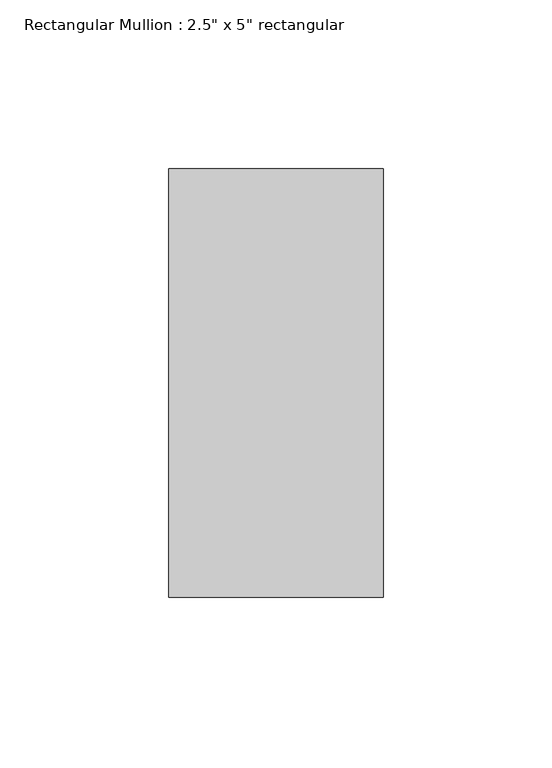
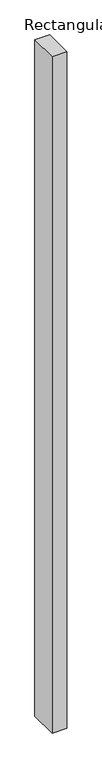
"""IFC4 building model written with IfcOpenShell, lengths in millimetres: member geometry."""

from ifc_helpers import new_model, si_unit, frame, origin, place, context, project, spatial, polyline, outline, extrude, source, transform, mapped, element, save


def member_eaba9652(model_context):
    return source(origin(), model_context, "Body", "SweptSolid", [
        extrude(outline(polyline([(31.75, 63.5), (31.75, -63.5), (-31.75, -63.5), (-31.75, 63.5), (31.75, 63.5)])), frame((0.0, 0.0, -3048.0), z_axis=(0.0, 0.0, 1.0), x_axis=(1.0, 0.0, 0.0)), (0.0, 0.0, 1.0), 3048.0),
    ])


if __name__ == "__main__":
    model = new_model("IFC4")
    model_context = context("Model", 3, world=origin())
    ifc_project = project(units=[si_unit("LENGTHUNIT", "METRE", prefix="MILLI")], contexts=[model_context])
    site = spatial("IfcSite", under=ifc_project)
    building = spatial("IfcBuilding", under=site)
    placement = place(None, origin())
    member_shape = member_eaba9652(model_context)
    element("IfcMember", 1, ObjectType="Rectangular Mullion : 2.5\" x 5\" rectangular", at=placement, inside=building, context=model_context, shape_type="MappedRepresentation", body=[
        mapped(member_shape, transform((0.0, 0.0, 0.0), x_axis=(1.0, 0.0, 0.0), y_axis=(0.0, 1.0, 0.0), z_axis=(0.0, 0.0, 1.0))),
    ])
    save(model, "model.ifc")

# Revit data of these elements
# Type "Rectangular Mullion : 2.5\" x 5\" rectangular"
#   built-in parameter 1007304 = 0.416667 (stored number, unit not read)
#   built-in parameter 1007301 = 0.104167 (stored number, unit not read)
#   built-in parameter 1007300 = 0.104167 (stored number, unit not read)
# Element 1 (IfcMember, "Rectangular Mullion : 2.5\" x 5\" rectangular")
#   Materials on its faces: "Aluminum"
# Materials
#   "Aluminum": class "Metal", colour RGB 247 247 247, transparency 0, Description = "Aluminum 6061", Cost = 0
